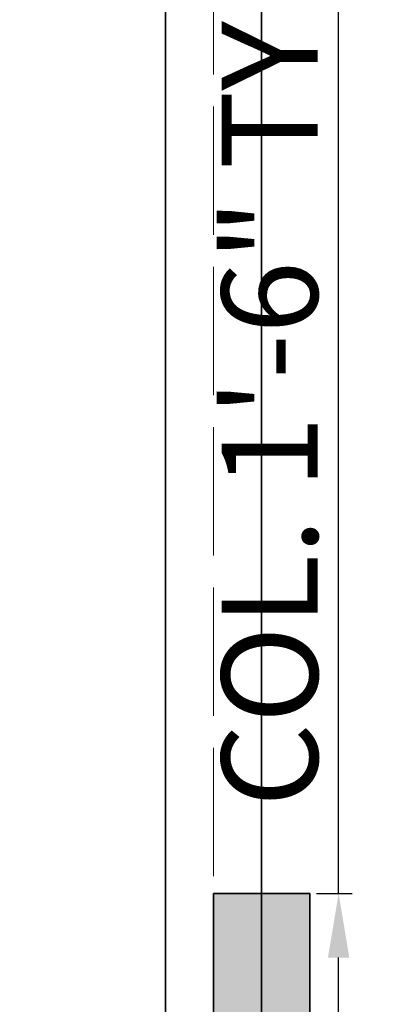
# Model space of a CAD drawing. Units: millimetres. Extents: x 595116 to 630915, y 909473 to 920225.
# Tile 114 of 134: x 629298 to 629331, y 919419 to 919512. Entities that reach past the tile are written whole.
import ezdxf

# ---------------------------------------------------------------- set-up
doc = ezdxf.new("R2010")
doc.units = ezdxf.units.MM
doc.linetypes.add('ACAD_ISO02W100', pattern=[15, 12, -3])
for name, color, linetype, lineweight in [('A-WALL', 1, 'Continuous', 35), ('C-PROP-REF', 240, 'ACAD_ISO02W100', 13), ('Column', 6, 'Continuous', 35), ('Dimension', 3, 'Continuous', 18)]:
    doc.layers.add(name, color=color, linetype=linetype, lineweight=lineweight)
doc.styles.get("Standard").update_dxf_attribs({"font": 'arial.ttf'})
doc.dimstyles.new('ISO-25', dxfattribs={"dimtxt": 9, "dimasz": 6, "dimexe": 1.25, "dimexo": 0.625, "dimtad": 1, "dimlunit": 4, "dimtxsty": 'Standard', "dimcen": 2.5, "dimadec": 0, "dimazin": 0, "dimtfac": 1, "dimtmove": 0, "dimatfit": 3, "dimfxl": 1, "dimarcsym": 0})

# ---------------------------------------------------------------- blocks, each defined once
blk = doc.blocks.new('*D128')
at = {"layer": 'Defpoints', "color": 0, "transparency": 16777216}
for p in [(629311.541, 920089.428), (629282.395, 919141.928), (629311.541, 919141.928)]:
    blk.add_point(p, dxfattribs=at)
at = {"layer": 'Dimension', "color": 0, "lineweight": -2, "transparency": 16777216}
for p, q in [((629310.916, 920089.428), (629281.145, 920089.428)), ((629282.395, 920083.428), (629282.395, 919147.928)), ((629310.916, 919141.928), (629281.145, 919141.928))]:
    blk.add_line(p, q, dxfattribs=at)
at = {"layer": 'Dimension', "color": 0, "transparency": 16777216}
for points in [[(629281.395, 920083.428), (629283.395, 920083.428), (629282.395, 920089.428)], [(629281.395, 919147.928), (629283.395, 919147.928), (629282.395, 919141.928)]]:
    blk.add_solid(points, dxfattribs=at)
at = {"layer": 'Dimension', "color": 0, "transparency": 16777216, "insert": (629271.157, 919615.678), "char_height": 9, "attachment_point": 5, "rotation": 90}
blk.add_mtext('78\'-11{\\H1x;\\S1/2;}"', dxfattribs=at)
blk = doc.blocks.new('COLUMN-RECT-9X18')
h = blk.add_hatch(color=256)
h.dxf.hatch_style = 1
h.paths.add_polyline_path([(9, 18), (0, 18), (0, 0), (9, 0)])
blk.add_lwpolyline([(0, 18), (9, 18), (9, 0), (0, 0)], close=True)
blk = doc.blocks.new('*D152')
at = {"layer": 'Defpoints', "color": 0, "transparency": 16777216}
for p in [(629325.041, 919429.828), (629327.741, 919429.828), (629325.041, 919411.828)]:
    blk.add_point(p, dxfattribs=at)
at = {"layer": 'Dimension', "color": 0, "lineweight": -2, "transparency": 16777216}
for p, q in [((629327.741, 919429.828), (629327.741, 919524.671)), ((629325.666, 919429.828), (629328.991, 919429.828)), ((629327.741, 919417.828), (629327.741, 919423.828)), ((629325.666, 919411.828), (629328.991, 919411.828))]:
    blk.add_line(p, q, dxfattribs=at)
at = {"layer": 'Dimension', "color": 0, "transparency": 16777216}
for points in [[(629326.741, 919423.828), (629328.741, 919423.828), (629327.741, 919429.828)], [(629326.741, 919417.828), (629328.741, 919417.828), (629327.741, 919411.828)]]:
    blk.add_solid(points, dxfattribs=at)
at = {"layer": 'Dimension', "color": 0, "transparency": 16777216, "insert": (629322.459, 919480.25), "char_height": 9, "attachment_point": 5, "rotation": 90}
blk.add_mtext('COL. 1\'-6" TYP.', dxfattribs=at)
blk = doc.blocks.new('*D153')
at = {"layer": 'Defpoints', "color": 0, "transparency": 16777216}
for p in [(629316.041, 919411.828), (629325.041, 919411.828), (629325.041, 919409.128)]:
    blk.add_point(p, dxfattribs=at)
at = {"layer": 'Dimension', "color": 0, "lineweight": -2, "transparency": 16777216}
for p, q in [((629316.041, 919411.203), (629316.041, 919407.878)), ((629325.041, 919411.203), (629325.041, 919407.878)), ((629310.041, 919409.128), (629304.041, 919409.128)), ((629316.041, 919409.128), (629325.041, 919409.128)), ((629331.041, 919409.128), (629393.15, 919409.128))]:
    blk.add_line(p, q, dxfattribs=at)
at = {"layer": 'Dimension', "color": 0, "transparency": 16777216}
for points in [[(629310.041, 919410.128), (629310.041, 919408.128), (629316.041, 919409.128)], [(629331.041, 919410.128), (629331.041, 919408.128), (629325.041, 919409.128)]]:
    blk.add_solid(points, dxfattribs=at)
at = {"layer": 'Dimension', "color": 0, "transparency": 16777216, "insert": (629365.096, 919414.348), "char_height": 9, "attachment_point": 5}
blk.add_mtext('0\'-9" TYP.', dxfattribs=at)

msp = doc.modelspace()

# ---------------------------------------------------------------- linework, layer by layer
at = {"layer": 'A-WALL'}
msp.add_line((629320.541, 919345.928), (629320.541, 919957.928), dxfattribs=at)
msp.add_lwpolyline([(629311.541, 919345.928), (629311.541, 919957.928)], dxfattribs=at)
at = {"layer": 'C-PROP-REF'}
msp.add_line((629316.041, 919146.428), (629316.041, 920084.928), dxfattribs=at)

# ---------------------------------------------------------------- block references
at = {"layer": 'Column'}
msp.add_blockref('COLUMN-RECT-9X18', (629316.041, 919411.828), dxfattribs=at)

# ---------------------------------------------------------------- dimensions: what is measured, and where the dimension line sits
at = {"layer": 'Dimension'}
dim = msp.add_linear_dim(base=(629282.395, 919141.928), p1=(629311.541, 920089.428), p2=(629311.541, 919141.928), angle=90, dimstyle='ISO-25', override={"dimclrd": 0, "dimclre": 0, "dimclrt": 0}, dxfattribs=at)
dim.commit()
dim.dimension.update_dxf_attribs({"geometry": '*D128', "text_midpoint": (629271.157, 919615.678)})
dim = msp.add_linear_dim(base=(629327.741, 919429.828), p1=(629325.041, 919411.828), p2=(629325.041, 919429.828), angle=90, text='COL. <> TYP.', dimstyle='ISO-25', override={"dimdec": 1, "dimlfac": 1, "dimrnd": 0, "dimzin": 1, "dimdsep": 46, "dimlunit": 4, "dimfrac": 2}, dxfattribs=at)
dim.commit()
dim.dimension.update_dxf_attribs({"geometry": '*D152', "text_midpoint": (629322.459, 919480.25)})
dim = msp.add_linear_dim(base=(629325.041, 919409.128), p1=(629316.041, 919411.828), p2=(629325.041, 919411.828), text='<> TYP.', dimstyle='ISO-25', override={"dimdec": 1, "dimlfac": 1, "dimrnd": 0, "dimzin": 1, "dimdsep": 46, "dimlunit": 4, "dimfrac": 2}, dxfattribs=at)
dim.commit()
dim.dimension.update_dxf_attribs({"geometry": '*D153', "text_midpoint": (629365.096, 919414.348)})

doc.saveas('drawing.dxf')
